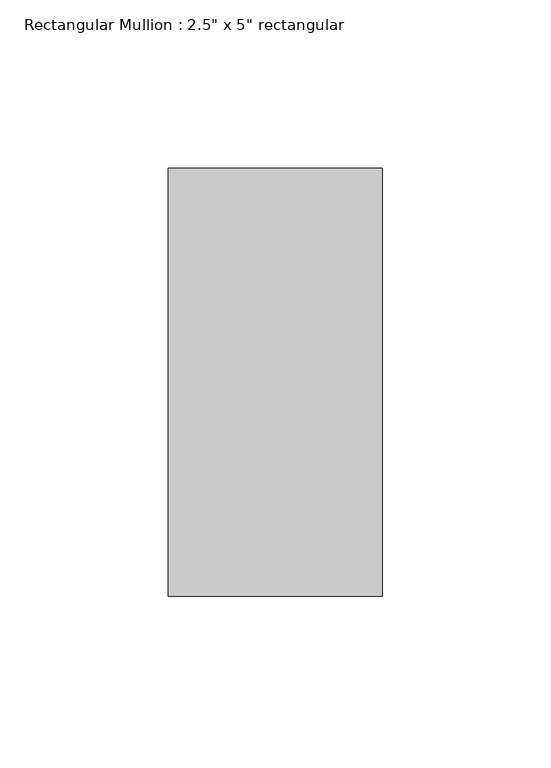
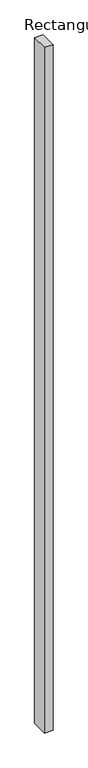
"""IFC4 building model written with IfcOpenShell, lengths in millimetres: member geometry."""

from ifc_helpers import new_model, si_unit, frame, origin, place, context, project, spatial, polyline, outline, extrude, source, transform, mapped, element, save


def member_ca7a94d5(model_context):
    return source(origin(), model_context, "Body", "SweptSolid", [
        extrude(outline(polyline([(0.0, 63.5), (0.0, -63.5), (-63.5, -63.5), (-63.5, 63.5), (0.0, 63.5)])), frame((0.0, 0.0, -5422.9), z_axis=(0.0, 0.0, 1.0), x_axis=(1.0, 0.0, 0.0)), (0.0, 0.0, 1.0), 5422.9),
    ])


if __name__ == "__main__":
    model = new_model("IFC4")
    model_context = context("Model", 3, world=origin())
    ifc_project = project(units=[si_unit("LENGTHUNIT", "METRE", prefix="MILLI")], contexts=[model_context])
    site = spatial("IfcSite", under=ifc_project)
    building = spatial("IfcBuilding", under=site)
    placement = place(None, origin())
    member_shape = member_ca7a94d5(model_context)
    element("IfcMember", 1, ObjectType="Rectangular Mullion : 2.5\" x 5\" rectangular", at=placement, inside=building, context=model_context, shape_type="MappedRepresentation", body=[
        mapped(member_shape, transform((0.0, 0.0, 0.0), x_axis=(1.0, 0.0, 0.0), y_axis=(0.0, 1.0, 0.0), z_axis=(0.0, 0.0, 1.0))),
    ])
    save(model, "model.ifc")

# Revit data of these elements
# Type "Rectangular Mullion : 2.5\" x 5\" rectangular"
#   built-in parameter 1007304 = 0.416667 (stored number, unit not read)
#   built-in parameter 1007301 = 0.104167 (stored number, unit not read)
#   built-in parameter 1007300 = 0.104167 (stored number, unit not read)
# Element 1 (IfcMember, "Rectangular Mullion : 2.5\" x 5\" rectangular")
#   Materials on its faces: "Aluminum"
# Materials
#   "Aluminum": class "Metal", colour RGB 247 247 247, transparency 0, Description = "Aluminum 6061", Cost = 0
